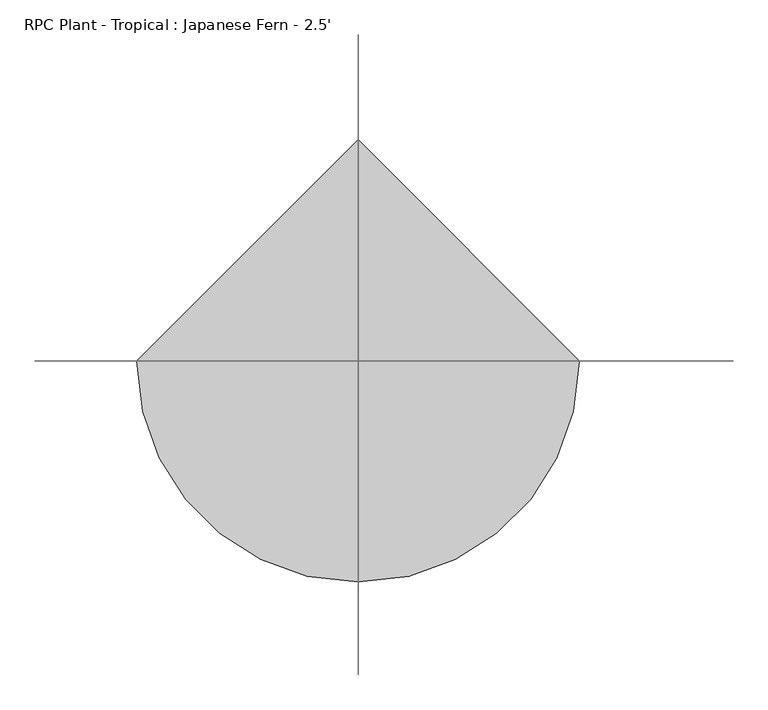
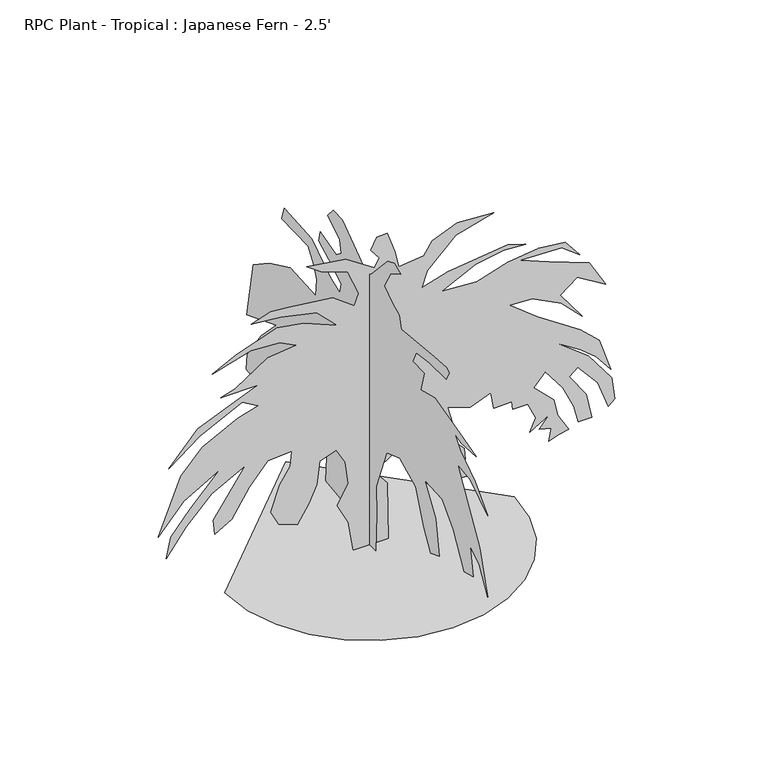
"""IFC4 building model written with IfcOpenShell, lengths in millimetres: geographic element geometry, RPC Plant - Tropical : Japanese Fern - 2.5'."""

from ifc_helpers import new_model, si_unit, origin, place, context, project, spatial, triangles, source, transform, mapped, element, save


def rpc_plant_tropical_japanese_fern_2_5_30b4c15b(model_context):
    return source(origin(), model_context, "Body", "Tessellation", [
        triangles([(-340.212337, 0.0, 2.34e-05), (-331.2181912, -77.9542988, 2.34e-05), (-305.6048564, -149.5428615, 2.34e-05), (-265.4195731, -212.7146324, 2.34e-05), (-212.7146324, -265.4195731, 2.34e-05), (-149.5428615, -305.6048564, 2.34e-05), (-77.9542988, -331.2181912, 2.34e-05), (1.49e-05, -340.212337, 2.34e-05), (77.9542988, -331.2181912, 2.34e-05), (149.5428615, -305.6048564, 2.34e-05), (212.7146324, -265.4195731, 2.34e-05), (265.4195731, -212.7146324, 2.34e-05), (305.6048564, -149.5428615, 2.34e-05), (331.2181912, -77.9542988, 2.34e-05), (340.212337, 2.97e-05, 2.34e-05), (-4.46e-05, 340.212337, 2.34e-05), (-37.8980319, 2.29e-05, 3.6e-06), (-50.0874814, 2.41e-05, 73.5418183), (-75.8826774, 2.22e-05, 123.7339445), (-49.5540792, 1.83e-05, 170.5209506), (-56.979003, 1.53e-05, 225.9335385), (-77.3492758, 1.4e-05, 262.2445852), (-116.2627981, 1.66e-05, 248.3474865), (-123.5028085, 2.02e-05, 192.7652324), (-143.0648503, 2.35e-05, 151.8270789), (-169.0734009, 2.72e-05, 109.3715308), (-213.7047246, 2.81e-05, 126.2541304), (-232.5443813, 2.67e-05, 163.0480237), (-210.7659323, 2.22e-05, 223.3318078), (-185.9735321, 1.89e-05, 260.6164324), (-182.3167059, 1.66e-05, 296.5396212), (-238.5613832, 1.93e-05, 292.8185184), (-282.7321973, 2.42e-05, 242.1521888), (-323.5728004, 2.99e-05, 177.126216), (-363.5396922, 3.3e-05, 153.4968807), (-367.1566226, 3.1e-05, 190.2732333), (-291.3732759, 2.12e-05, 298.3785896), (-370.9310652, 2.72e-05, 256.7835813), (-430.3492407, 3.34e-05, 195.5366293), (-477.8725754, 3.92e-05, 133.2528402), (-467.4636904, 3.58e-05, 182.8625483), (-420.8344145, 3.05e-05, 237.2243282), (-351.5280344, 2.32e-05, 310.1438599), (-436.732245, 2.98e-05, 261.3606638), (-497.0571965, 3.65e-05, 192.7571115), (-443.5089389, 2.62e-05, 326.4709519), (-392.9096655, 2.08e-05, 380.0648827), (-309.8949288, 1.46e-05, 423.094996), (-260.7967811, 1.16e-05, 437.3545544), (-299.3412489, 1.2e-05, 459.500768), (-398.9192914, 1.93e-05, 409.5872812), (-471.8705798, 2.58e-05, 354.6903414), (-403.1941031, 1.83e-05, 430.1180775), (-300.6061608, 1.12e-05, 473.1100754), (-262.5823916, 8.7e-06, 488.4237482), (-349.0058046, 1.24e-05, 488.2357873), (-315.6607106, 1.04e-05, 498.3805169), (-238.5613832, 4e-06, 548.5353044), (-172.4069002, 6e-07, 556.9452561), (-210.7659323, 1.1e-06, 576.3305191), (-278.7875798, 3.9e-06, 580.4732532), (-369.1987945, 9.4e-06, 554.0953574), (-313.0699167, 5.2e-06, 582.9446503), (-216.6861742, -1e-06, 616.0738781), (-154.0988607, -3.1e-06, 605.5227053), (-75.0741966, -4.5e-06, 572.1420393), (-123.4916265, -5.3e-06, 620.6382071), (-209.0953766, -2.7e-06, 638.8728498), (-277.4743968, -1e-07, 645.8171934), (-232.2393309, -3e-06, 661.5423237), (-190.0088236, -4.6e-06, 657.7145777), (-85.7208487, -8.4e-06, 644.6056395), (-35.6564855, -8.3e-06, 606.9044523), (-24.5384073, -1.05e-05, 634.6996307), (-50.8667489, -1.3e-05, 696.1980572), (-113.4009815, -1.16e-05, 718.2401711), (-146.8372491, -1.16e-05, 743.1016623), (-55.5814956, -1.48e-05, 730.2366045), (11.5952668, -1.5e-05, 684.7325506), (23.1518731, -1.68e-05, 706.0913486), (3.2567592, -1.75e-05, 731.9840996), (17.6289544, -1.97e-05, 758.3441912), (41.4979712, -2.09e-05, 760.5615704), (59.6452374, -1.86e-05, 708.9971306), (68.5156716, -1.65e-05, 668.0955574), (127.4710438, -1.95e-05, 674.2321741), (147.7915331, -2.21e-05, 704.1889212), (206.1616894, -2.62e-05, 729.2028013), (292.3257614, -2.96e-05, 723.6452917), (202.8348031, -2.42e-05, 698.6847513), (136.1791696, -1.75e-05, 634.3440565), (123.7575623, -1.46e-05, 595.466851), (183.9252741, -1.84e-05, 615.2432602), (325.6810292, -2.56e-05, 631.9208759), (367.486835, -2.67e-05, 619.3809437), (315.6911957, -2.46e-05, 622.1876038), (249.7079049, -2.1e-05, 609.8203354), (170.7500609, -1.52e-05, 570.6967787), (252.258585, -1.85e-05, 566.1527246), (325.6530876, -2.3e-05, 588.2608592), (397.9490381, -2.68e-05, 598.5656445), (460.1815041, -2.91e-05, 591.0853598), (495.2309272, -2.81e-05, 548.5353044), (452.9501141, -2.81e-05, 580.5189626), (355.0433722, -2.4e-05, 583.2977174), (420.1841635, -2.53e-05, 556.8741122), (516.8336057, -2.73e-05, 520.4505724), (556.2848313, -2.51e-05, 453.460657), (489.3051261, -2.46e-05, 494.41557), (449.4220591, -2.1e-05, 463.6816175), (500.7909802, -1.9e-05, 392.8817239), (450.7580967, -1.98e-05, 442.9146074), (383.0951119, -1.89e-05, 477.7430411), (329.99392, -1.68e-05, 480.9358332), (395.1677399, -1.66e-05, 429.0157465), (495.6652757, -1.69e-05, 361.8734422), (541.06265, -1.64e-05, 319.2167072), (567.5802175, -1.27e-05, 237.3833302), (533.9328526, -1.38e-05, 280.9008592), (497.6007317, -1.4e-05, 310.7127932), (440.194243, -1.36e-05, 346.6664852), (514.6872977, -1.35e-05, 290.0397636), (570.595186, -1.15e-05, 215.9856355), (576.6531012, -8.5e-06, 161.5684811), (561.938883, -7.1e-06, 148.2847988), (536.9249665, -1e-05, 214.9932542), (489.6734176, -1.12e-05, 270.583393), (469.5464848, -9.4e-06, 254.0962635), (510.5775922, -7.7e-06, 195.5264555), (523.0261056, -4.6e-06, 134.3872005), (491.7079591, -3.2e-06, 133.6020922), (481.1339315, -5.3e-06, 176.3159639), (454.7662096, -7.4e-06, 231.6510674), (413.5344604, -8.8e-06, 285.1248746), (386.501263, -5.8e-06, 255.5745526), (434.0830244, -5.2e-06, 209.4342185), (443.1813063, -3e-06, 166.6068182), (468.6523896, -1.6e-06, 123.9640722), (446.3842358, -3e-07, 118.289464), (421.5049404, 1.3e-06, 110.591996), (428.004798, -8e-07, 139.9015351), (399.5416008, 0.0, 147.6790127), (422.9629183, -2.7e-06, 176.0799863), (377.2150203, 9e-07, 148.592647), (391.2256476, -1.5e-06, 179.1531272), (372.9656067, -3.1e-06, 218.8891102), (336.6588839, -1.5e-06, 219.0854463), (334.8783603, -2.6e-06, 238.301043), (292.3257614, -6e-07, 237.2294151), (285.8309907, -2.8e-06, 277.7512695), (236.7361495, 5e-07, 259.4658122), (183.9252741, 1.8e-06, 276.1434461), (200.6023993, 4.7e-06, 214.9932542), (199.418242, 6.4e-06, 187.1818159), (222.8385421, 6.9e-06, 162.1823971), (225.6180599, 8.4e-06, 134.3872005), (208.5548754, 9.9e-06, 121.5754553), (237.8440942, 1.05e-05, 90.4480402), (182.0385615, 1.28e-05, 92.8412262), (191.5158174, 1e-05, 133.3458033), (165.4579784, 1e-05, 152.2179799), (173.5882597, 8.2e-06, 176.3515177), (109.0494575, 1.14e-05, 169.6062899), (94.9809212, 1.06e-05, 192.7571115), (145.0122605, 6.8e-06, 220.5522899), (83.3228392, 9.3e-06, 223.7369429), (11.6764698, 1.52e-05, 177.2189248), (42.170055, 1.61e-05, 139.9462362), (44.9495728, 1.82e-05, 0.0), (0.00212, 26.6938489, 3.6e-06), (0.0021253, 22.2078332, 125.235588), (0.0021271, 60.1697466, 128.8281648), (0.002126, 119.4035039, 42.9622804), (0.0021289, 177.9956579, 51.1230378), (0.0021314, 173.4581986, 113.1355544), (0.0021337, 137.5657583, 202.421547), (0.0021299, 136.57414, 252.5593115), (0.0021317, 167.407932, 262.8744886), (0.0021371, 226.3958104, 190.2732333), (0.0021373, 288.3557457, 133.4656906), (0.0021388, 315.632769, 140.3605096), (0.0021407, 309.8923854, 190.0641981), (0.0021433, 346.6360002, 212.5124464), (0.0021443, 409.4094941, 172.1231784), (0.0021442, 453.2701527, 125.235588), (0.0021466, 501.6723581, 132.7981805), (0.0021481, 497.133391, 172.1231784), (0.0021432, 441.1721629, 252.2857635), (0.0021433, 378.8939512, 316.9053294), (0.0021465, 498.6472157, 270.4360728), (0.0021515, 472.2337844, 410.5144049), (0.0021506, 407.8956694, 453.4479761), (0.0021486, 323.1969149, 492.7747544), (0.0021437, 217.6417118, 487.9487409), (0.0021455, 214.2957677, 530.5851645), (0.0021473, 226.9167634, 559.1017015), (0.0021497, 249.3380874, 591.8626016), (0.0021545, 357.9821463, 594.1105021), (0.0021554, 347.3954378, 625.8731346), (0.0021502, 235.3830889, 618.7560545), (0.0021449, 161.3091401, 570.0389337), (0.0021424, 119.7014417, 554.0699593), (0.0021433, 115.4461873, 579.5537599), (0.0021468, 165.8956152, 609.2361777), (0.0021495, 206.7331843, 630.4121017), (0.0021444, 199.1706008, 657.6358034), (0.0021408, 134.2553771, 640.0184195), (0.0021406, 114.4705746, 656.1245584), (0.0021422, 120.4276329, 685.149095), (0.0021457, 170.4330744, 716.6247173), (0.0021458, 147.7455603, 742.3371014), (0.0021442, 111.4454322, 740.823313), (0.002139, 41.6899925, 691.1155186), (0.0021365, 10.7464246, 665.9695244), (0.0021362, -10.1176737, 680.5009048), (0.0021365, -74.5923583, 749.8987038), (0.0021358, -101.8173226, 761.9992733), (0.0021341, -127.5299701, 749.8987038), (0.0021349, -87.1447716, 726.4240465), (0.002134, -60.7928054, 680.9606152), (0.0021316, -92.5270285, 657.5951809), (0.0021298, -121.8045655, 644.2526087), (0.0021341, -129.7537351, 615.210268), (0.0021228, -265.1681168, 628.8983133), (0.0021208, -315.0816035, 631.9234194), (0.00212, -325.668312, 624.3618896), (0.0021255, -313.5677788, 601.6746117), (0.0021285, -243.6485001, 600.9557965), (0.0021305, -191.8444855, 593.8259992), (0.0021298, -176.5968879, 563.282551), (0.0021277, -223.3409642, 562.4341653), (0.0021262, -209.0156213, 512.3124063), (0.0021243, -266.6794162, 527.5625656), (0.0021188, -366.5470304, 501.9288832), (0.002115, -434.5681692, 482.1855025), (0.0021175, -375.2998755, 480.0595058), (0.002119, -348.4190672, 487.3848581), (0.0021168, -370.0115719, 459.7014462), (0.0021124, -430.801357, 418.7795254), (0.0021078, -482.9678312, 365.7240792), (0.0021129, -410.4102324, 411.3017841), (0.0021154, -360.3773852, 417.8549815), (0.0021108, -398.4519507, 351.1901917), (0.0021049, -449.6938448, 265.8970875), (0.0021049, -481.8349789, 162.1823971), (0.002103, -448.18002, 222.0356478), (0.0021056, -410.473746, 244.4529204), (0.0021022, -423.4226649, 177.6834858), (0.0021093, -387.3318446, 167.7414328), (0.0021087, -342.3053052, 246.2357331), (0.0021128, -296.4634267, 293.7202257), (0.0021161, -226.1207364, 298.3785896), (0.0021111, -271.2183834, 229.5982494), (0.0021128, -284.3374772, 144.5642138), (0.0021137, -249.3695898, 130.0336417), (0.002117, -221.7963819, 179.3619262), (0.002116, -188.1828268, 259.1153067), (0.0021202, -123.9887073, 290.1007337), (0.0021217, -70.0716722, 271.1447323), (0.0021248, -27.498267, 162.3606929), (0.0021217, -30.4360283, 94.6027103), (0.0021177, -25.7012178, 2.43e-05)], [[15, 16, 1], [14, 15, 1], [14, 1, 2], [13, 14, 2], [13, 2, 3], [13, 3, 4], [12, 13, 4], [11, 12, 4], [11, 4, 5], [11, 5, 6], [11, 6, 7], [11, 7, 8], [11, 8, 9], [11, 9, 10], [110, 111, 112], [51, 52, 53], [61, 62, 63], [102, 103, 104], [94, 95, 96], [55, 56, 57], [88, 89, 90], [44, 45, 46], [117, 118, 119], [61, 63, 64], [68, 69, 70], [39, 40, 41], [107, 108, 109], [76, 77, 78], [39, 41, 42], [75, 76, 78], [38, 39, 42], [38, 42, 43], [60, 61, 64], [143, 144, 145], [93, 94, 96], [93, 96, 97], [93, 97, 98], [68, 70, 71], [37, 38, 43], [55, 57, 58], [157, 158, 159], [157, 159, 160], [75, 78, 79], [92, 93, 98], [74, 75, 79], [67, 68, 71], [67, 71, 72], [110, 112, 113], [139, 140, 141], [87, 88, 90], [87, 90, 91], [86, 87, 91], [117, 119, 120], [116, 117, 120], [116, 120, 121], [115, 116, 121], [101, 102, 104], [101, 104, 105], [100, 101, 105], [106, 107, 109], [34, 35, 36], [141, 142, 143], [43, 44, 46], [43, 46, 47], [124, 125, 126], [123, 124, 126], [122, 123, 126], [122, 126, 127], [34, 36, 37], [33, 34, 37], [32, 33, 37], [60, 64, 65], [59, 60, 65], [137, 138, 139], [137, 139, 141], [137, 141, 143], [136, 137, 143], [121, 122, 127], [50, 51, 53], [50, 53, 54], [66, 67, 72], [66, 72, 73], [106, 109, 110], [106, 110, 113], [129, 130, 131], [129, 131, 132], [129, 132, 133], [128, 129, 133], [128, 133, 134], [43, 47, 48], [37, 43, 48], [105, 106, 113], [105, 113, 114], [100, 105, 114], [99, 100, 114], [59, 65, 66], [163, 164, 165], [162, 163, 165], [168, 169, 17], [168, 17, 18], [168, 18, 19], [168, 19, 20], [167, 168, 20], [167, 20, 21], [146, 147, 148], [121, 127, 128], [121, 128, 134], [85, 86, 91], [148, 149, 150], [37, 48, 49], [32, 37, 49], [31, 32, 49], [85, 91, 92], [25, 26, 27], [25, 27, 28], [25, 28, 29], [24, 25, 29], [24, 29, 30], [23, 24, 30], [23, 30, 31], [136, 143, 145], [135, 136, 145], [135, 145, 146], [135, 146, 148], [82, 83, 84], [81, 82, 84], [80, 81, 84], [80, 84, 85], [79, 80, 85], [50, 54, 55], [49, 50, 55], [160, 161, 162], [156, 157, 160], [155, 156, 160], [155, 160, 162], [154, 155, 162], [154, 162, 165], [153, 154, 165], [152, 153, 165], [74, 79, 85], [74, 85, 92], [73, 74, 92], [166, 167, 21], [55, 58, 59], [166, 21, 22], [152, 165, 166], [135, 148, 150], [134, 135, 150], [121, 134, 150], [115, 121, 150], [114, 115, 150], [114, 150, 151], [114, 151, 152], [99, 114, 152], [98, 99, 152], [98, 152, 166], [98, 166, 22], [92, 98, 22], [73, 92, 22], [66, 73, 22], [59, 66, 22], [55, 59, 22], [49, 55, 22], [31, 49, 22], [23, 31, 22], [244, 245, 246], [239, 240, 241], [234, 235, 236], [234, 236, 237], [233, 234, 237], [238, 239, 241], [238, 241, 242], [217, 218, 219], [216, 217, 219], [189, 190, 191], [244, 246, 247], [215, 216, 219], [215, 219, 220], [197, 198, 199], [197, 199, 200], [230, 231, 232], [189, 191, 192], [209, 210, 211], [209, 211, 212], [209, 212, 213], [208, 209, 213], [197, 200, 201], [196, 197, 201], [195, 196, 201], [243, 244, 247], [262, 170, 171], [261, 262, 171], [260, 261, 171], [205, 206, 207], [204, 205, 207], [203, 204, 207], [185, 186, 187], [184, 185, 187], [184, 187, 188], [183, 184, 188], [183, 188, 189], [173, 174, 175], [172, 173, 175], [172, 175, 176], [247, 248, 249], [247, 249, 250], [243, 247, 250], [243, 250, 251], [242, 243, 251], [254, 255, 256], [253, 254, 256], [253, 256, 257], [252, 253, 257], [225, 226, 227], [224, 225, 227], [224, 227, 228], [223, 224, 228], [223, 228, 229], [223, 229, 230], [180, 181, 182], [179, 180, 182], [189, 192, 193], [189, 193, 194], [252, 257, 258], [203, 207, 208], [242, 251, 252], [208, 213, 214], [203, 208, 214], [183, 189, 194], [182, 183, 194], [179, 182, 194], [178, 179, 194], [177, 178, 194], [195, 201, 202], [194, 195, 202], [177, 194, 202], [237, 238, 242], [237, 242, 252], [233, 237, 252], [232, 233, 252], [232, 252, 258], [230, 232, 258], [230, 258, 259], [223, 230, 259], [221, 222, 223], [221, 223, 259], [220, 221, 259], [215, 220, 259], [214, 215, 259], [203, 214, 259], [202, 203, 259], [177, 202, 259], [177, 259, 260], [176, 177, 260], [172, 176, 260], [172, 260, 171]], closed=False),
    ])


if __name__ == "__main__":
    model = new_model("IFC4")
    model_context = context("Model", 3, world=origin())
    ifc_project = project(units=[si_unit("LENGTHUNIT", "METRE", prefix="MILLI")], contexts=[model_context])
    site = spatial("IfcSite", under=ifc_project)
    building = spatial("IfcBuilding", under=site)
    placement = place(None, origin())
    rpc_plant_tropical_japanese_fern_2_5_shape = rpc_plant_tropical_japanese_fern_2_5_30b4c15b(model_context)
    element("IfcGeographicElement", 1, ObjectType="RPC Plant - Tropical : Japanese Fern - 2.5'", at=placement, inside=building, context=model_context, shape_type="MappedRepresentation", body=[
        mapped(rpc_plant_tropical_japanese_fern_2_5_shape, transform((0.0, 0.0, 0.0), x_axis=(1.0, 0.0, 0.0), y_axis=(0.0, 1.0, 0.0), z_axis=(0.0, 0.0, 1.0))),
    ])
    save(model, "model.ifc")

# Revit data of these elements
# Type "RPC Plant - Tropical : Japanese Fern - 2.5'"
#   built-in parameter 1005198 = "{2, 15},{39, RPC-16-G1GK-JAPX-7J4P-Q000-ST1L-LVER-AU},{1, 0},{1, 0},{2, 35},{1, 8},{5, Color},{1, 0},{1, 0},{3, 0.8},{3, 0.8},{3, 0.8},{1, 8},{7, BBoxMin},{1, 0},{1, 0},{1, 0},{1, 0},{1, 0},{1, 8},{7, BBoxMax},{1, 0},{1, 0},{1, 0},{1, 0},{1, 0},{2, 11},{9, RPCTypeId},{1, 0},{1, 0},{39, RPC-16-G1GK-JAPX-7J4P-Q000-ST1L-LVER-AU},{1, 6},{14, RPCPlantHeight},{1, 0},{1, 0},{3, 2.5},{2, 11},{7, keyword},{1, 0},{1, 0},{53, :Geometry:RPC:Japanese Fern:plant:small:japanese fern},{2, 11},{8, category},{1, 0},{1, 0},{17, :Shrubs [General]},{2, 11},{12, LocalizedUID},{1, 0},{1, 0},{13, Japanese Fern},{2, 14},{6, Height},{1, 0},{1, 0},{3, 2.5},{1, 2},{16, Cast Reflections},{1, 0},{1, 0},{1, 0},{1, 2},{12, Cast Shadows},{1, 0},{1, 0},{1, 1},{1, 2},{9, Lock View},{1, 0},{1, 0},{1, 0},{1, 4},{5, ViewC},{1, 0},{1, 0},{1, 0},{2, 11},{20, AdvancedUIDefinition},{1, 0},{1, 0},{0, },{2, 11},{10, AssetLibID},{1, 0},{1, 0},{36, 4D3F6E72-3F99-4203-98E9-AF80B3C7A7A4},{2, 11},{10, BaseSchema},{1, 0},{1, 0},{9, RPCSchema},{2, 11},{12, ExchangeGUID},{1, 0},{1, 0},{0, },{1, 2},{6, Hidden},{1, 0},{1, 0},{1, 0},{1, 4},{11, RPCCategory},{1, 0},{1, 0},{1, 0},{2, 11},{8, RPCImage},{1, 0},{1, 0},{0, },{1, 4},{13, SchemaVersion},{1, 0},{1, 0},{1, 4},{2, 11},{12, UIDefinition},{1, 0},{1, 0},{0, },{2, 11},{6, UIName},{1, 0},{1, 0},{39, RPC-16-G1GK-JAPX-7J4P-Q000-ST1L-LVER-AU},{2, 11},{11, VersionGUID},{1, 0},{1, 0},{9, RPCSchema},{2, 11},{9, assettype},{1, 0},{1, 0},{11, RPCGeometry},{2, 11},{11, description},{1, 0},{1, 0},{0, },{2, 11},{9, localname},{1, 0},{1, 0},{3, RPC},{2, 11},{9, localtype},{1, 0},{1, 0},{3, RPC},{1, 4},{8, revision},{1, 0},{1, 0},{1, 1},{2, 11},{9, thumbnail},{1, 0},{1, 0},{0, },{1, 4},{7, version},{1, 0},{1, 0},{1, 1},{1, 2},{20, RPC_Cast Reflections},{1, 0},{1, 0},{1, 1},{1, 2},{16, RPC_Cast Shadows},{1, 0},{1, 0},{1, 1},{1, 2},{13, RPC_Lock View},{1, 0},{1, 0},{1, 0},{1, 4},{9, RPC_ViewC},{1, 0},{1, 0},{1, 0},{21, assetlibrary_base.fbx},{1, 5},"
#   built-in parameter 1005195 = "RPC-16-G1GK-JAPX-7J4P-Q000-ST1L-LVER-AU"
#   Type Comments = "Japanese Fern"
#   Assembly Code = "G2050500"
#   Height = 2' - 6"
#   Default Elevation = 0
